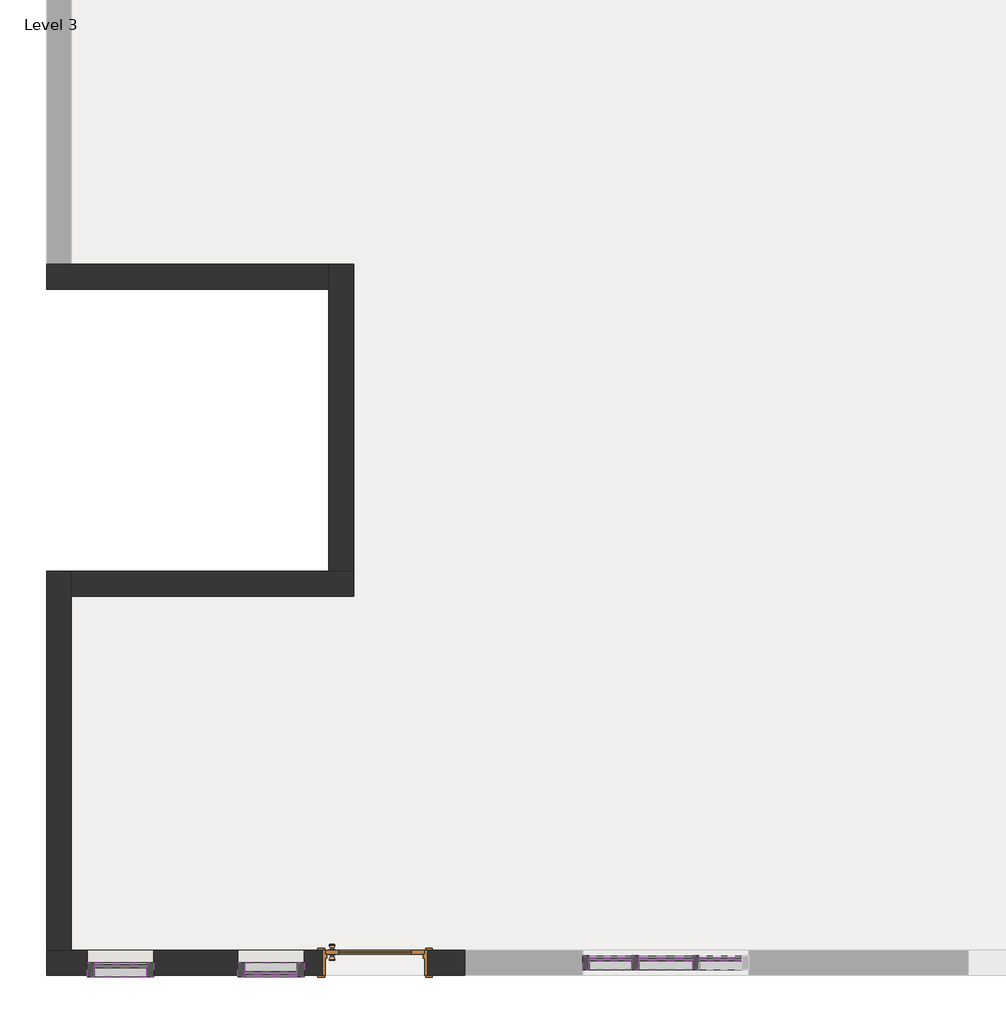
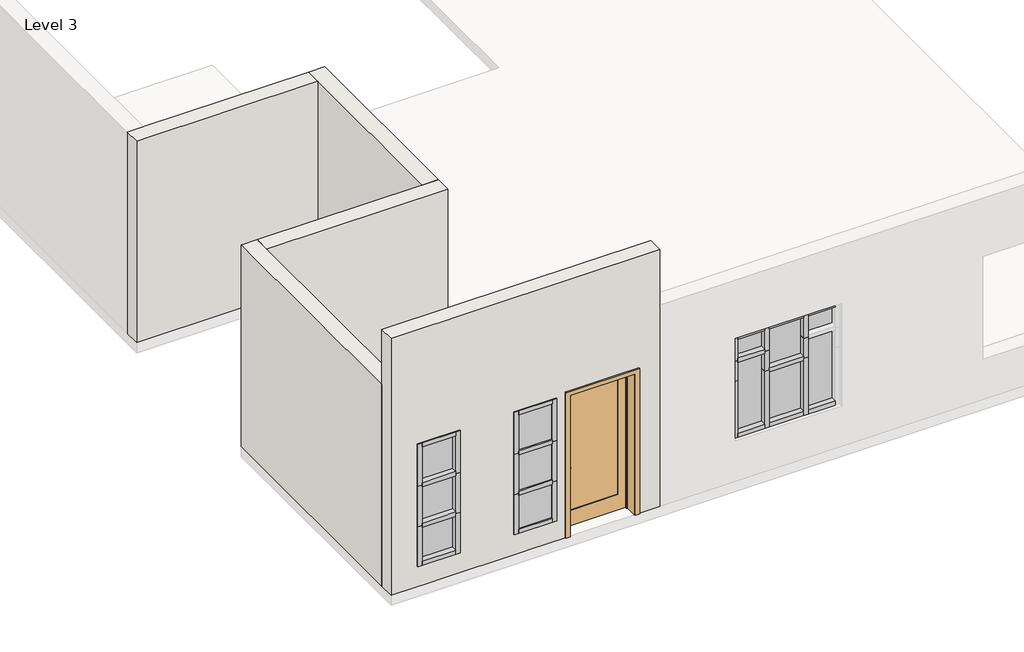
# One storey, part 1 of 2: 37 members, 12 plates, 5 walls, 1 door.
"""IFC4 building model written with IfcOpenShell, lengths in millimetres."""

from ifc_helpers import new_model, si_unit, origin, place, context, project, spatial, faceted_brep, transform, mapped, element, save
from components import door_3b97b8e7, member_86d06fe4, member_323df77c, member_47bfaf8a, member_5e365d0c, member_dffdf235, member_fd92426f, member_3709dd30, member_9ab3e039, member_2ebf4a73, member_75d1e245, member_3c3dc66a, member_b70ee1cc, member_03a502dc, member_dfe75557, system_panel_glazed_c43f0a09, system_panel_glazed_07c93182, system_panel_glazed_2a04ea5f, system_panel_glazed_e6031cb5, system_panel_glazed_9dd6121d, system_panel_glazed_7704e2d2, system_panel_glazed_d8783796

model = new_model("IFC4")

# Units and contexts
model_context = context("Model", 3, world=origin())
ifc_project = project(units=[si_unit("LENGTHUNIT", "METRE", prefix="MILLI")], contexts=[model_context])

# Site, building, storey
site = spatial("IfcSite", under=ifc_project)
building = spatial("IfcBuilding", under=site)
storey = spatial("IfcBuildingStorey", under=building, Name="Level 3", Elevation=3810.0)

# Door
placement = place(None, origin())
door_shape = door_3b97b8e7(model_context)
element("IfcDoor", 1, ObjectType="Door-Interior-Single-1_Panel-Wood : 36\" x 84\"", at=placement, inside=storey, context=model_context, shape_type="MappedRepresentation", body=[
    mapped(door_shape, transform((-9143.1179297, 32.0946292, 3810.0), x_axis=(1.0, 0.0, 0.0), y_axis=(0.0, 1.0, 0.0), z_axis=(0.0, 0.0, 1.0))),
])

# Members
member_shape = member_86d06fe4(model_context)
element("IfcMember", 2, ObjectType="Rectangular Mullion : 2.5\" x 5\" rectangular", at=placement, inside=storey, context=model_context, shape_type="MappedRepresentation", body=[
    mapped(member_shape, transform((-10341.5348984, -34.5803708, 5969.0), x_axis=(0.0, 0.0, 1.0), y_axis=(0.0, 1.0, 0.0), z_axis=(-1.0, 0.0, 0.0))),
])
element("IfcMember", 3, ObjectType="Rectangular Mullion : 2.5\" x 5\" rectangular", at=placement, inside=storey, context=model_context, shape_type="MappedRepresentation", body=[
    mapped(member_shape, transform((-11238.6179297, -34.5803708, 5969.0), x_axis=(0.0, 0.0, 1.0), y_axis=(0.0, -1.0, 0.0), z_axis=(1.0, 0.0, 0.0))),
])
element("IfcMember", 4, ObjectType="Rectangular Mullion : 2.5\" x 5\" rectangular", at=placement, inside=storey, context=model_context, shape_type="MappedRepresentation", body=[
    mapped(member_shape, transform((-9858.9348984, -34.5803708, 4114.8), x_axis=(0.0, 0.0, -1.0), y_axis=(0.0, 1.0, 0.0), z_axis=(1.0, 0.0, 0.0))),
])
element("IfcMember", 5, ObjectType="Rectangular Mullion : 2.5\" x 5\" rectangular", at=placement, inside=storey, context=model_context, shape_type="MappedRepresentation", body=[
    mapped(member_shape, transform((-11721.2179297, -34.5803708, 4114.8), x_axis=(0.0, 0.0, -1.0), y_axis=(0.0, -1.0, 0.0), z_axis=(-1.0, 0.0, 0.0))),
])
member_2_shape = member_323df77c(model_context)
element("IfcMember", 6, ObjectType="Rectangular Mullion : 2.5\" x 5\" rectangular", at=placement, inside=storey, context=model_context, shape_type="MappedRepresentation", body=[
    mapped(member_2_shape, transform((-10341.5348984, -34.5803708, 5334.0), x_axis=(0.0, 0.0, 1.0), y_axis=(0.0, 1.0, 0.0), z_axis=(-1.0, 0.0, 0.0))),
])
element("IfcMember", 7, ObjectType="Rectangular Mullion : 2.5\" x 5\" rectangular", at=placement, inside=storey, context=model_context, shape_type="MappedRepresentation", body=[
    mapped(member_2_shape, transform((-10341.5348984, -34.5803708, 4724.4), x_axis=(0.0, 0.0, 1.0), y_axis=(0.0, 1.0, 0.0), z_axis=(-1.0, 0.0, 0.0))),
])
element("IfcMember", 8, ObjectType="Rectangular Mullion : 2.5\" x 5\" rectangular", at=placement, inside=storey, context=model_context, shape_type="MappedRepresentation", body=[
    mapped(member_2_shape, transform((-11238.6179297, -34.5803708, 5334.0), x_axis=(0.0, 0.0, 1.0), y_axis=(0.0, -1.0, 0.0), z_axis=(1.0, 0.0, 0.0))),
])
element("IfcMember", 9, ObjectType="Rectangular Mullion : 2.5\" x 5\" rectangular", at=placement, inside=storey, context=model_context, shape_type="MappedRepresentation", body=[
    mapped(member_2_shape, transform((-11238.6179297, -34.5803708, 4724.4), x_axis=(0.0, 0.0, 1.0), y_axis=(0.0, -1.0, 0.0), z_axis=(1.0, 0.0, 0.0))),
])
member_3_shape = member_47bfaf8a(model_context)
element("IfcMember", 10, ObjectType="Rectangular Mullion : 2.5\" x 5\" rectangular", at=placement, inside=storey, context=model_context, shape_type="MappedRepresentation", body=[
    mapped(member_3_shape, transform((-10405.0348984, -34.5803708, 4114.8), x_axis=(-1.0, 0.0, 0.0), y_axis=(0.0, 1.0, 0.0), z_axis=(0.0, 0.0, -1.0))),
])
element("IfcMember", 11, ObjectType="Rectangular Mullion : 2.5\" x 5\" rectangular", at=placement, inside=storey, context=model_context, shape_type="MappedRepresentation", body=[
    mapped(member_3_shape, transform((-11175.1179297, -34.5803708, 4114.8), x_axis=(1.0, 0.0, 0.0), y_axis=(0.0, -1.0, 0.0), z_axis=(0.0, 0.0, -1.0))),
])
element("IfcMember", 12, ObjectType="Rectangular Mullion : 2.5\" x 5\" rectangular", at=placement, inside=storey, context=model_context, shape_type="MappedRepresentation", body=[
    mapped(member_3_shape, transform((-10405.0348984, -34.5803708, 4724.4), x_axis=(-1.0, 0.0, 0.0), y_axis=(0.0, 1.0, 0.0), z_axis=(0.0, 0.0, -1.0))),
])
element("IfcMember", 13, ObjectType="Rectangular Mullion : 2.5\" x 5\" rectangular", at=placement, inside=storey, context=model_context, shape_type="MappedRepresentation", body=[
    mapped(member_3_shape, transform((-11175.1179297, -34.5803708, 4724.4), x_axis=(1.0, 0.0, 0.0), y_axis=(0.0, -1.0, 0.0), z_axis=(0.0, 0.0, -1.0))),
])
element("IfcMember", 14, ObjectType="Rectangular Mullion : 2.5\" x 5\" rectangular", at=placement, inside=storey, context=model_context, shape_type="MappedRepresentation", body=[
    mapped(member_3_shape, transform((-9795.4348984, -34.5803708, 5334.0), x_axis=(1.0, 0.0, 0.0), y_axis=(0.0, 1.0, 0.0), z_axis=(0.0, 0.0, 1.0))),
])
element("IfcMember", 15, ObjectType="Rectangular Mullion : 2.5\" x 5\" rectangular", at=placement, inside=storey, context=model_context, shape_type="MappedRepresentation", body=[
    mapped(member_3_shape, transform((-11784.7179297, -34.5803708, 5334.0), x_axis=(-1.0, 0.0, 0.0), y_axis=(0.0, -1.0, 0.0), z_axis=(0.0, 0.0, 1.0))),
])
element("IfcMember", 16, ObjectType="Rectangular Mullion : 2.5\" x 5\" rectangular", at=placement, inside=storey, context=model_context, shape_type="MappedRepresentation", body=[
    mapped(member_3_shape, transform((-9795.4348984, -34.5803708, 4724.4), x_axis=(1.0, 0.0, 0.0), y_axis=(0.0, 1.0, 0.0), z_axis=(0.0, 0.0, 1.0))),
])
element("IfcMember", 17, ObjectType="Rectangular Mullion : 2.5\" x 5\" rectangular", at=placement, inside=storey, context=model_context, shape_type="MappedRepresentation", body=[
    mapped(member_3_shape, transform((-11784.7179297, -34.5803708, 4724.4), x_axis=(-1.0, 0.0, 0.0), y_axis=(0.0, -1.0, 0.0), z_axis=(0.0, 0.0, 1.0))),
])
member_4_shape = member_5e365d0c(model_context)
element("IfcMember", 18, ObjectType="Rectangular Mullion : 2.5\" x 5\" rectangular", at=placement, inside=storey, context=model_context, shape_type="MappedRepresentation", body=[
    mapped(member_4_shape, transform((-9795.4348984, -34.5803708, 5969.0), x_axis=(1.0, 0.0, 0.0), y_axis=(0.0, 1.0, 0.0), z_axis=(0.0, 0.0, 1.0))),
])
element("IfcMember", 19, ObjectType="Rectangular Mullion : 2.5\" x 5\" rectangular", at=placement, inside=storey, context=model_context, shape_type="MappedRepresentation", body=[
    mapped(member_4_shape, transform((-11784.7179297, -34.5803708, 5969.0), x_axis=(-1.0, 0.0, 0.0), y_axis=(0.0, -1.0, 0.0), z_axis=(0.0, 0.0, 1.0))),
])
element("IfcMember", 20, ObjectType="Rectangular Mullion : 2.5\" x 5\" rectangular", at=placement, inside=storey, context=model_context, shape_type="MappedRepresentation", body=[
    mapped(member_4_shape, transform((-10405.0348984, -34.5803708, 5334.0), x_axis=(-1.0, 0.0, 0.0), y_axis=(0.0, 1.0, 0.0), z_axis=(0.0, 0.0, -1.0))),
])
element("IfcMember", 21, ObjectType="Rectangular Mullion : 2.5\" x 5\" rectangular", at=placement, inside=storey, context=model_context, shape_type="MappedRepresentation", body=[
    mapped(member_4_shape, transform((-11175.1179297, -34.5803708, 5334.0), x_axis=(1.0, 0.0, 0.0), y_axis=(0.0, -1.0, 0.0), z_axis=(0.0, 0.0, -1.0))),
])
member_5_shape = member_dffdf235(model_context)
element("IfcMember", 22, ObjectType="Rectangular Mullion : 2.5\" x 5\" rectangular", at=placement, inside=storey, context=model_context, shape_type="MappedRepresentation", body=[
    mapped(member_5_shape, transform((-5777.6179297, 28.9196292, 5969.0), x_axis=(0.0, 0.0, 1.0), y_axis=(0.0, -1.0, 0.0), z_axis=(1.0, 0.0, 0.0))),
])
element("IfcMember", 23, ObjectType="Rectangular Mullion : 2.5\" x 5\" rectangular", at=placement, inside=storey, context=model_context, shape_type="MappedRepresentation", body=[
    mapped(member_5_shape, transform((-6787.2679297, 28.9196292, 5969.0), x_axis=(0.0, 0.0, 1.0), y_axis=(0.0, -1.0, 0.0), z_axis=(1.0, 0.0, 0.0))),
])
element("IfcMember", 24, ObjectType="Rectangular Mullion : 2.5\" x 5\" rectangular", at=placement, inside=storey, context=model_context, shape_type="MappedRepresentation", body=[
    mapped(member_5_shape, transform((-7174.6179297, 28.9196292, 4419.6), x_axis=(0.0, 0.0, -1.0), y_axis=(0.0, -1.0, 0.0), z_axis=(-1.0, 0.0, 0.0))),
])
element("IfcMember", 25, ObjectType="Rectangular Mullion : 2.5\" x 5\" rectangular", at=placement, inside=storey, context=model_context, shape_type="MappedRepresentation", body=[
    mapped(member_5_shape, transform((-6164.9679297, 28.9196292, 4419.6), x_axis=(0.0, 0.0, -1.0), y_axis=(0.0, -1.0, 0.0), z_axis=(-1.0, 0.0, 0.0))),
])
member_6_shape = member_fd92426f(model_context)
element("IfcMember", 26, ObjectType="Rectangular Mullion : 2.5\" x 5\" rectangular", at=placement, inside=storey, context=model_context, shape_type="MappedRepresentation", body=[
    mapped(member_6_shape, transform((-6755.5179297, 28.9196292, 4419.6), x_axis=(1.0, 0.0, 0.0), y_axis=(0.0, -1.0, 0.0), z_axis=(0.0, 0.0, -1.0))),
])
element("IfcMember", 27, ObjectType="Rectangular Mullion : 2.5\" x 5\" rectangular", at=placement, inside=storey, context=model_context, shape_type="MappedRepresentation", body=[
    mapped(member_6_shape, transform((-6196.7179297, 28.9196292, 4419.6), x_axis=(1.0, 0.0, 0.0), y_axis=(0.0, -1.0, 0.0), z_axis=(0.0, 0.0, -1.0))),
])
member_7_shape = member_3709dd30(model_context)
element("IfcMember", 28, ObjectType="Rectangular Mullion : 2.5\" x 5\" rectangular", at=placement, inside=storey, context=model_context, shape_type="MappedRepresentation", body=[
    mapped(member_7_shape, transform((-6787.2679297, 28.9196292, 5588.0), x_axis=(0.0, 0.0, 1.0), y_axis=(0.0, -1.0, 0.0), z_axis=(1.0, 0.0, 0.0))),
])
member_8_shape = member_9ab3e039(model_context)
element("IfcMember", 29, ObjectType="Rectangular Mullion : 2.5\" x 5\" rectangular", at=placement, inside=storey, context=model_context, shape_type="MappedRepresentation", body=[
    mapped(member_8_shape, transform((-6228.4679297, 28.9196292, 5283.2), x_axis=(0.0, 0.0, 1.0), y_axis=(0.0, -1.0, 0.0), z_axis=(1.0, 0.0, 0.0))),
])
member_9_shape = member_2ebf4a73(model_context)
element("IfcMember", 30, ObjectType="Rectangular Mullion : 2.5\" x 5\" rectangular", at=placement, inside=storey, context=model_context, shape_type="MappedRepresentation", body=[
    mapped(member_9_shape, transform((-6723.7679297, 28.9196292, 4419.6), x_axis=(0.0, 0.0, -1.0), y_axis=(0.0, -1.0, 0.0), z_axis=(-1.0, 0.0, 0.0))),
])
element("IfcMember", 31, ObjectType="Rectangular Mullion : 2.5\" x 5\" rectangular", at=placement, inside=storey, context=model_context, shape_type="MappedRepresentation", body=[
    mapped(member_9_shape, transform((-6228.4679297, 28.9196292, 5969.0), x_axis=(0.0, 0.0, 1.0), y_axis=(0.0, -1.0, 0.0), z_axis=(1.0, 0.0, 0.0))),
])
member_10_shape = member_75d1e245(model_context)
element("IfcMember", 32, ObjectType="Rectangular Mullion : 2.5\" x 5\" rectangular", at=placement, inside=storey, context=model_context, shape_type="MappedRepresentation", body=[
    mapped(member_10_shape, transform((-6755.5179297, 28.9196292, 5283.2), x_axis=(1.0, 0.0, 0.0), y_axis=(0.0, -1.0, 0.0), z_axis=(0.0, 0.0, -1.0))),
])
element("IfcMember", 33, ObjectType="Rectangular Mullion : 2.5\" x 5\" rectangular", at=placement, inside=storey, context=model_context, shape_type="MappedRepresentation", body=[
    mapped(member_10_shape, transform((-6196.7179297, 28.9196292, 5283.2), x_axis=(1.0, 0.0, 0.0), y_axis=(0.0, -1.0, 0.0), z_axis=(0.0, 0.0, -1.0))),
])
member_11_shape = member_3c3dc66a(model_context)
element("IfcMember", 34, ObjectType="Rectangular Mullion : 2.5\" x 5\" rectangular", at=placement, inside=storey, context=model_context, shape_type="MappedRepresentation", body=[
    mapped(member_11_shape, transform((-7238.1179297, 28.9196292, 5588.0), x_axis=(-1.0, 0.0, 0.0), y_axis=(0.0, -1.0, 0.0), z_axis=(0.0, 0.0, 1.0))),
])
member_12_shape = member_b70ee1cc(model_context)
element("IfcMember", 35, ObjectType="Rectangular Mullion : 2.5\" x 5\" rectangular", at=placement, inside=storey, context=model_context, shape_type="MappedRepresentation", body=[
    mapped(member_12_shape, transform((-7238.1179297, 28.9196292, 5283.2), x_axis=(-1.0, 0.0, 0.0), y_axis=(0.0, -1.0, 0.0), z_axis=(0.0, 0.0, 1.0))),
])
member_13_shape = member_03a502dc(model_context)
element("IfcMember", 36, ObjectType="Rectangular Mullion : 2.5\" x 5\" rectangular", at=placement, inside=storey, context=model_context, shape_type="MappedRepresentation", body=[
    mapped(member_13_shape, transform((-6755.5179297, 28.9196292, 5588.0), x_axis=(1.0, 0.0, 0.0), y_axis=(0.0, -1.0, 0.0), z_axis=(0.0, 0.0, -1.0))),
])
element("IfcMember", 37, ObjectType="Rectangular Mullion : 2.5\" x 5\" rectangular", at=placement, inside=storey, context=model_context, shape_type="MappedRepresentation", body=[
    mapped(member_13_shape, transform((-6196.7179297, 28.9196292, 5588.0), x_axis=(1.0, 0.0, 0.0), y_axis=(0.0, -1.0, 0.0), z_axis=(0.0, 0.0, -1.0))),
])
member_14_shape = member_dfe75557(model_context)
element("IfcMember", 38, ObjectType="Rectangular Mullion : 2.5\" x 5\" rectangular", at=placement, inside=storey, context=model_context, shape_type="MappedRepresentation", body=[
    mapped(member_14_shape, transform((-7238.1179297, 28.9196292, 5969.0), x_axis=(-1.0, 0.0, 0.0), y_axis=(0.0, -1.0, 0.0), z_axis=(0.0, 0.0, 1.0))),
])

# Plates
system_panel_glazed_shape = system_panel_glazed_c43f0a09(model_context)
element("IfcPlate", 39, ObjectType="System Panel : Glazed", at=placement, inside=storey, context=model_context, shape_type="MappedRepresentation", body=[
    mapped(system_panel_glazed_shape, transform((-10100.2348984, -34.5803708, 4178.3), x_axis=(-1.0, 0.0, 0.0), y_axis=(0.0, -1.0, 0.0), z_axis=(0.0, 0.0, 1.0))),
])
element("IfcPlate", 40, ObjectType="System Panel : Glazed", at=placement, inside=storey, context=model_context, shape_type="MappedRepresentation", body=[
    mapped(system_panel_glazed_shape, transform((-11479.9179297, -34.5803708, 4178.3), x_axis=(1.0, 0.0, 0.0), y_axis=(0.0, 1.0, 0.0), z_axis=(0.0, 0.0, 1.0))),
])
system_panel_glazed_2_shape = system_panel_glazed_07c93182(model_context)
element("IfcPlate", 41, ObjectType="System Panel : Glazed", at=placement, inside=storey, context=model_context, shape_type="MappedRepresentation", body=[
    mapped(system_panel_glazed_2_shape, transform((-11479.9179297, -34.5803708, 4756.15), x_axis=(1.0, 0.0, 0.0), y_axis=(0.0, 1.0, 0.0), z_axis=(0.0, 0.0, 1.0))),
])
element("IfcPlate", 42, ObjectType="System Panel : Glazed", at=placement, inside=storey, context=model_context, shape_type="MappedRepresentation", body=[
    mapped(system_panel_glazed_2_shape, transform((-10100.2348984, -34.5803708, 4756.15), x_axis=(-1.0, 0.0, 0.0), y_axis=(0.0, -1.0, 0.0), z_axis=(0.0, 0.0, 1.0))),
])
system_panel_glazed_3_shape = system_panel_glazed_2a04ea5f(model_context)
element("IfcPlate", 43, ObjectType="System Panel : Glazed", at=placement, inside=storey, context=model_context, shape_type="MappedRepresentation", body=[
    mapped(system_panel_glazed_3_shape, transform((-11479.9179297, -34.5803708, 5365.75), x_axis=(1.0, 0.0, 0.0), y_axis=(0.0, 1.0, 0.0), z_axis=(0.0, 0.0, 1.0))),
])
element("IfcPlate", 44, ObjectType="System Panel : Glazed", at=placement, inside=storey, context=model_context, shape_type="MappedRepresentation", body=[
    mapped(system_panel_glazed_3_shape, transform((-10100.2348984, -34.5803708, 5365.75), x_axis=(-1.0, 0.0, 0.0), y_axis=(0.0, -1.0, 0.0), z_axis=(0.0, 0.0, 1.0))),
])
system_panel_glazed_4_shape = system_panel_glazed_e6031cb5(model_context)
element("IfcPlate", 45, ObjectType="System Panel : Glazed", at=placement, inside=storey, context=model_context, shape_type="MappedRepresentation", body=[
    mapped(system_panel_glazed_4_shape, transform((-6980.9429297, 28.9196292, 4483.1), x_axis=(1.0, 0.0, 0.0), y_axis=(0.0, 1.0, 0.0), z_axis=(0.0, 0.0, 1.0))),
])
element("IfcPlate", 46, ObjectType="System Panel : Glazed", at=placement, inside=storey, context=model_context, shape_type="MappedRepresentation", body=[
    mapped(system_panel_glazed_4_shape, transform((-5971.2929297, 28.9196292, 4483.1), x_axis=(1.0, 0.0, 0.0), y_axis=(0.0, 1.0, 0.0), z_axis=(0.0, 0.0, 1.0))),
])
system_panel_glazed_5_shape = system_panel_glazed_9dd6121d(model_context)
element("IfcPlate", 47, ObjectType="System Panel : Glazed", at=placement, inside=storey, context=model_context, shape_type="MappedRepresentation", body=[
    mapped(system_panel_glazed_5_shape, transform((-6476.1179297, 28.9196292, 4483.1), x_axis=(1.0, 0.0, 0.0), y_axis=(0.0, 1.0, 0.0), z_axis=(0.0, 0.0, 1.0))),
])
system_panel_glazed_6_shape = system_panel_glazed_7704e2d2(model_context)
element("IfcPlate", 48, ObjectType="System Panel : Glazed", at=placement, inside=storey, context=model_context, shape_type="MappedRepresentation", body=[
    mapped(system_panel_glazed_6_shape, transform((-6980.9429297, 28.9196292, 5619.75), x_axis=(1.0, 0.0, 0.0), y_axis=(0.0, 1.0, 0.0), z_axis=(0.0, 0.0, 1.0))),
])
element("IfcPlate", 49, ObjectType="System Panel : Glazed", at=placement, inside=storey, context=model_context, shape_type="MappedRepresentation", body=[
    mapped(system_panel_glazed_6_shape, transform((-5971.2929297, 28.9196292, 5619.75), x_axis=(1.0, 0.0, 0.0), y_axis=(0.0, 1.0, 0.0), z_axis=(0.0, 0.0, 1.0))),
])
system_panel_glazed_7_shape = system_panel_glazed_d8783796(model_context)
element("IfcPlate", 50, ObjectType="System Panel : Glazed", at=placement, inside=storey, context=model_context, shape_type="MappedRepresentation", body=[
    mapped(system_panel_glazed_7_shape, transform((-6476.1179297, 28.9196292, 5314.95), x_axis=(1.0, 0.0, 0.0), y_axis=(0.0, 1.0, 0.0), z_axis=(0.0, 0.0, 1.0))),
])

# Walls
element("IfcWall", 51, ObjectType="9\" wall", at=placement, inside=storey, context=model_context, shape_type="Brep", body=[
    faceted_brep([(-11930.7679297, 143.2196292, 3810.0), (-11930.7679297, 3394.4196292, 3810.0), (-11930.7679297, 3623.0196292, 3810.0), (-11930.7679297, 3623.0196292, 6858.0), (-11930.7679297, 3394.4196292, 6858.0), (-11930.7679297, 143.2196292, 6858.0), (-12159.3679297, 143.2196292, 3810.0), (-12159.3679297, 143.2196292, 6858.0), (-12159.3679297, 3623.0196292, 6858.0), (-12159.3679297, 3623.0196292, 3810.0)], [[[0, 1, 2, 3, 4, 5]], [[6, 7, 8, 9]], [[2, 1, 0, 6, 9]], [[5, 4, 3, 8, 7]], [[0, 5, 7, 6]], [[3, 2, 9, 8]]]),
])
element("IfcWall", 52, ObjectType="9\" wall", at=placement, inside=storey, context=model_context, shape_type="Brep", body=[
    faceted_brep([(-11930.7679297, 3394.4196292, 3810.0), (-9339.9679297, 3394.4196292, 3810.0), (-9339.9679297, 3394.4196292, 6858.0), (-11930.7679297, 3394.4196292, 6858.0), (-11930.7679297, 3623.0196292, 3810.0), (-11930.7679297, 3623.0196292, 6858.0), (-9568.5679297, 3623.0196292, 6858.0), (-9339.9679297, 3623.0196292, 6858.0), (-9339.9679297, 3623.0196292, 3810.0), (-9568.5679297, 3623.0196292, 3810.0)], [[[0, 1, 2, 3]], [[4, 5, 6, 7, 8, 9]], [[1, 0, 4, 9, 8]], [[3, 2, 7, 6, 5]], [[0, 3, 5, 4]], [[2, 1, 8, 7]]]),
])
element("IfcWall", 53, ObjectType="9\" wall", at=placement, inside=storey, context=model_context, shape_type="Brep", body=[
    faceted_brep([(-9339.9679297, 3623.0196292, 3810.0), (-9339.9679297, 6442.4196292, 3810.0), (-9339.9679297, 6442.4196292, 6858.0), (-9339.9679297, 3623.0196292, 6858.0), (-9568.5679297, 3623.0196292, 3810.0), (-9568.5679297, 3623.0196292, 6858.0), (-9568.5679297, 6213.8196292, 6858.0), (-9568.5679297, 6442.4196292, 6858.0), (-9568.5679297, 6442.4196292, 3810.0), (-9568.5679297, 6213.8196292, 3810.0)], [[[0, 1, 2, 3]], [[4, 5, 6, 7, 8, 9]], [[1, 0, 4, 9, 8]], [[3, 2, 7, 6, 5]], [[0, 3, 5, 4]], [[2, 1, 8, 7]]]),
])
element("IfcWall", 54, ObjectType="9\" wall", at=placement, inside=storey, context=model_context, shape_type="Brep", body=[
    faceted_brep([(-9568.5679297, 6442.4196292, 3810.0), (-11930.7679297, 6442.4196292, 3810.0), (-12159.3679297, 6442.4196292, 3810.0), (-12159.3679297, 6442.4196292, 6858.0), (-11930.7679297, 6442.4196292, 6858.0), (-9568.5679297, 6442.4196292, 6858.0), (-9568.5679297, 6213.8196292, 3810.0), (-9568.5679297, 6213.8196292, 6858.0), (-12159.3679297, 6213.8196292, 6858.0), (-12159.3679297, 6213.8196292, 3810.0)], [[[0, 1, 2, 3, 4, 5]], [[6, 7, 8, 9]], [[2, 1, 0, 6, 9]], [[5, 4, 3, 8, 7]], [[0, 5, 7, 6]], [[3, 2, 9, 8]]]),
])
element("IfcWall", 55, ObjectType="9\" wall", at=placement, inside=storey, context=model_context, shape_type="Brep", body=[
    faceted_brep([(-12159.3679297, 143.2196292, 7692.4706735), (-8317.6179297, 143.2196292, 7692.4706735), (-8317.6179297, 143.2196292, 6858.0), (-8317.6179297, 143.2196292, 3810.0), (-8660.5179297, 143.2196292, 3810.0), (-8660.5179297, 143.2196292, 5969.0), (-9625.7179297, 143.2196292, 5969.0), (-9625.7179297, 143.2196292, 3810.0), (-11930.7679297, 143.2196292, 3810.0), (-12159.3679297, 143.2196292, 3810.0), (-12159.3679297, 143.2196292, 6858.0), (-9795.4348984, 143.2196292, 4114.8), (-9795.4348984, 143.2196292, 5969.0), (-10405.0348984, 143.2196292, 5969.0), (-10405.0348984, 143.2196292, 4114.8), (-11784.7179297, 143.2196292, 5969.0), (-11784.7179297, 143.2196292, 4114.8), (-11175.1179297, 143.2196292, 4114.8), (-11175.1179297, 143.2196292, 5969.0), (-8317.6179297, -85.3803708, 7692.4706735), (-12159.3679297, -85.3803708, 7692.4706735), (-12159.3679297, -85.3803708, 3810.0), (-9625.7179297, -85.3803708, 3810.0), (-9625.7179297, -85.3803708, 5969.0), (-8660.5179297, -85.3803708, 5969.0), (-8660.5179297, -85.3803708, 3810.0), (-8317.6179297, -85.3803708, 3810.0), (-8317.6179297, -85.3803708, 6858.0), (-9795.4348984, -85.3803708, 5969.0), (-9795.4348984, -85.3803708, 4114.8), (-10405.0348984, -85.3803708, 4114.8), (-10405.0348984, -85.3803708, 5969.0), (-11784.7179297, -85.3803708, 4114.8), (-11784.7179297, -85.3803708, 5969.0), (-11175.1179297, -85.3803708, 5969.0), (-11175.1179297, -85.3803708, 4114.8)], [[[0, 1, 2, 3, 4, 5, 6, 7, 8, 9, 10], [11, 12, 13, 14], [15, 16, 17, 18]], [[19, 20, 21, 22, 23, 24, 25, 26, 27], [28, 29, 30, 31], [32, 33, 34, 35]], [[21, 9, 8, 7, 22]], [[3, 26, 25, 4]], [[1, 0, 20, 19]], [[3, 2, 1, 19, 27, 26]], [[0, 10, 9, 21, 20]], [[24, 5, 4, 25]], [[5, 24, 23, 6]], [[6, 23, 22, 7]], [[11, 29, 28, 12]], [[12, 28, 31, 13]], [[13, 31, 30, 14]], [[29, 11, 14, 30]], [[32, 16, 15, 33]], [[33, 15, 18, 34]], [[34, 18, 17, 35]], [[16, 32, 35, 17]]]),
])

save(model, "model.ifc")

# Revit data of these elements
# Type "Door-Interior-Single-1_Panel-Wood : 36\" x 84\""
#   Type Mark = "8"
#   Assembly Code = "C1020300"
#   Analytic Construction = "Wooden"
#   Top Rail = 0' - 4 11/16"
#   Thickness = 0' - 1 3/8"
#   Thermal Resistance (R) = 2.5876 (h·ft²·°F)/BTU
#   Swing Angle [instance default] = 90.00°
#   Stiles = 0' - 4 3/4"
#   Rough Width = 3' - 2"
#   Rough Height = 7' - 1"
#   Height = 7' - 0"
#   Width = 3' - 0"
#   Heat Transfer Coefficient (U) = 0.3865 BTU/(h·ft²·°F)
#   Bottom Rail = 0' - 9 1/8"
#   Panel Material = door colour
#   Frame Material = door colour
#   Door Handle Material = door colour
#   Visual Light Transmittance = 0
#   Solar Heat Gain Coefficient = 0
#   Wall Closure = (empty or 0)
#   Function = (empty or 0)
# Type "Rectangular Mullion : 2.5\" x 5\" rectangular"
#   built-in parameter 1007304 = 0.416667 (stored number, unit not read)
#   built-in parameter 1007301 = 0.104167 (stored number, unit not read)
#   built-in parameter 1007300 = 0.104167 (stored number, unit not read)
# Type "System Panel : Glazed"
#   Construction Type Id = "GSP4R"
#   Analytic Construction = "1/8 in Pilkington single glazing"
#   Visual Light Transmittance = 0.9
#   Solar Heat Gain Coefficient = 0.86
#   Heat Transfer Coefficient (U) = 1.18115 BTU/(h·ft²·°F)
#   Define Thermal Properties by = 1
# Type "9\" wall"
#   Assembly Code = "B2010"
#   Layers, outside or top first: 0' - 9" "Laminate, Ivory, Matte" (function 1)
# Element 1 (IfcDoor, "Door-Interior-Single-1_Panel-Wood : 36\" x 84\"")
#   Swing Angle = 90.00°
#   Phase Created = New Construction
#   Materials on its faces: "door colour"
# Elements 2, 3, 4, 5, 6, 7, 8, 9, 10, 11, 12, 13, 14, 15, 16, 17, 18, 19, 20, 21, 22, 23, 24, 25, 26, 27, 28, 29, 30, 31, 32, 33, 34, 35, 36, 37, 38 (IfcMember, "Rectangular Mullion : 2.5\" x 5\" rectangular")
#   Phase Created = New Construction
#   Materials on its faces: "door colour"
# Elements 39, 40, 41, 42, 43, 44, 45, 46, 47, 48, 49, 50 (IfcPlate, "System Panel : Glazed")
#   Phase Created = New Construction
#   Materials on its faces: "Glass"
# Elements 51, 52, 53, 54 (IfcWall, "9\" wall")
#   Top Offset = 0' - 0"
#   Base Offset = 0' - 0"
#   wall height = 10' - 0"
#   Phase Created = New Construction
#   Base Constraint = Level 3
#   Top Constraint = Level 4
#   Materials on its faces: "Laminate, Ivory, Matte"
# Element 55 (IfcWall, "9\" wall")
#   Top Offset = 2' - 8.85318"
#   Base Offset = 0' - 0"
#   wall height = 12' - 8.85318"
#   Phase Created = New Construction
#   Base Constraint = Level 3
#   Top Constraint = Level 4
#   Materials on its faces: "Laminate, Ivory, Matte"
# Materials
#   "door colour": class "Generic", colour RGB 120 120 120, transparency 0, Cost = 0
#   "Laminate, Ivory, Matte": class "Plastic", colour RGB 247 247 239, transparency 0, Description = "Plastic Laminate - Ivory, Matte", Cost = 0
#   "Glass": class "Glass", colour RGB 0 128 192, transparency 0.75, Description = "Soda Lime Glass", Cost = 0
